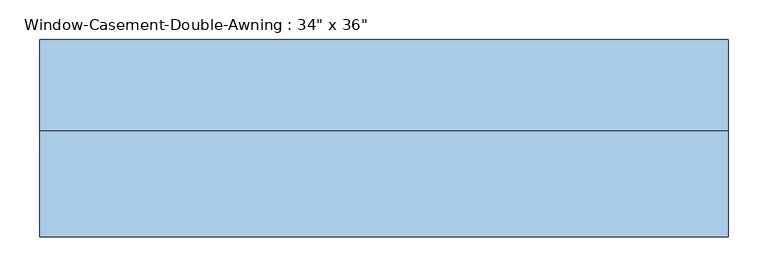
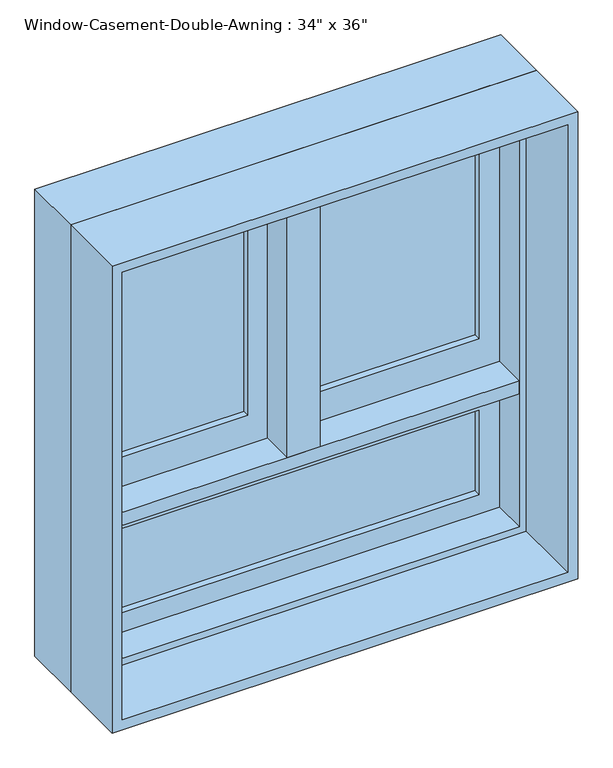
"""IFC4 building model written with IfcOpenShell, lengths in millimetres: window geometry."""

from ifc_helpers import new_model, si_unit, frame, origin, place, context, project, spatial, polyline, outline, extrude, faceted_brep, source, transform, mapped, element, save


def window_ced37e8f(model_context):
    return source(origin(), model_context, "Body", "SolidModel", [
        faceted_brep([(400.05, 82.55, 1797.05), (400.05, 19.05, 1797.05), (-400.05, 19.05, 1797.05), (-400.05, 82.55, 1797.05), (419.1, 133.35, 1816.1), (419.1, 82.55, 1816.1), (-419.1, 82.55, 1816.1), (-419.1, 133.35, 1816.1), (431.8, 19.05, 1828.8), (431.8, 133.35, 1828.8), (-431.8, 133.35, 1828.8), (-431.8, 19.05, 1828.8), (-400.05, 19.05, 946.15), (-400.05, 82.55, 946.15), (-419.1, 82.55, 927.1), (-419.1, 133.35, 927.1), (-431.8, 133.35, 914.4), (-431.8, 19.05, 914.4), (400.05, 19.05, 946.15), (400.05, 82.55, 946.15), (419.1, 82.55, 927.1), (419.1, 133.35, 927.1), (431.8, 133.35, 914.4), (431.8, 19.05, 914.4)], [[[0, 1, 2, 3]], [[4, 5, 6, 7]], [[8, 9, 10, 11]], [[3, 2, 12, 13]], [[7, 6, 14, 15]], [[11, 10, 16, 17]], [[13, 12, 18, 19]], [[15, 14, 20, 21]], [[17, 16, 22, 23]], [[11, 17, 23, 8], [1, 18, 12, 2]], [[19, 18, 1, 0]], [[5, 20, 14, 6], [3, 13, 19, 0]], [[21, 20, 5, 4]], [[23, 22, 9, 8]], [[9, 22, 16, 10], [7, 15, 21, 4]]]),
        extrude(outline(polyline([(1231.9, 419.1), (1816.1, 419.1), (1816.1, 9.525), (1231.9, 9.525), (1231.9, 419.1)]), holes=[polyline([(1289.05, 66.675), (1758.95, 66.675), (1758.95, 361.95), (1289.05, 361.95), (1289.05, 66.675)])]), frame((0.0, 82.55, 0.0), z_axis=(0.0, 1.0, 0.0), x_axis=(0.0, 0.0, 1.0)), (0.0, 0.0, 1.0), 44.45),
        extrude(outline(polyline([(1816.1, -419.1), (1231.9, -419.1), (1231.9, -9.525), (1816.1, -9.525), (1816.1, -419.1)]), holes=[polyline([(1758.95, -66.675), (1289.05, -66.675), (1289.05, -361.95), (1758.95, -361.95), (1758.95, -66.675)])]), frame((0.0, 82.55, 0.0), z_axis=(0.0, 1.0, 0.0), x_axis=(0.0, 0.0, 1.0)), (0.0, 0.0, 1.0), 44.45),
        extrude(outline(polyline([(361.95, 114.3), (361.95, 107.95), (66.675, 107.95), (66.675, 114.3), (361.95, 114.3)])), frame((0.0, 0.0, 1289.05), z_axis=(0.0, 0.0, 1.0), x_axis=(1.0, 0.0, 0.0)), (0.0, 0.0, 1.0), 469.9),
        extrude(outline(polyline([(66.675, 95.25), (66.675, 101.6), (361.95, 101.6), (361.95, 95.25), (66.675, 95.25)])), frame((0.0, 0.0, 1289.05), z_axis=(0.0, 0.0, 1.0), x_axis=(1.0, 0.0, 0.0)), (0.0, 0.0, 1.0), 469.9),
        extrude(outline(polyline([(-66.675, 114.3), (-66.675, 107.95), (-361.95, 107.95), (-361.95, 114.3), (-66.675, 114.3)])), frame((0.0, 0.0, 1289.05), z_axis=(0.0, 0.0, 1.0), x_axis=(1.0, 0.0, 0.0)), (0.0, 0.0, 1.0), 469.9),
        extrude(outline(polyline([(-361.95, 95.25), (-361.95, 101.6), (-66.675, 101.6), (-66.675, 95.25), (-361.95, 95.25)])), frame((0.0, 0.0, 1289.05), z_axis=(0.0, 0.0, 1.0), x_axis=(1.0, 0.0, 0.0)), (0.0, 0.0, 1.0), 469.9),
        extrude(outline(polyline([(400.05, 19.05), (-400.05, 19.05), (-400.05, 82.55), (-419.1, 82.55), (-419.1, 133.35), (419.1, 133.35), (419.1, 82.55), (400.05, 82.55), (400.05, 19.05)])), frame((0.0, 0.0, 1206.5), z_axis=(0.0, 0.0, 1.0), x_axis=(1.0, 0.0, 0.0)), (0.0, 0.0, 1.0), 25.4),
        extrude(outline(polyline([(1206.5, -419.1), (927.1, -419.1), (927.1, 419.1), (1206.5, 419.1), (1206.5, -419.1)]), holes=[polyline([(1149.35, 361.95), (984.25, 361.95), (984.25, -361.95), (1149.35, -361.95), (1149.35, 361.95)])]), frame((0.0, 82.55, 0.0), z_axis=(0.0, 1.0, 0.0), x_axis=(0.0, 0.0, 1.0)), (0.0, 0.0, 1.0), 44.45),
        extrude(outline(polyline([(361.95, 114.3), (361.95, 107.95), (-361.95, 107.95), (-361.95, 114.3), (361.95, 114.3)])), frame((0.0, 0.0, 984.25), z_axis=(0.0, 0.0, 1.0), x_axis=(1.0, 0.0, 0.0)), (0.0, 0.0, 1.0), 165.1),
        extrude(outline(polyline([(361.95, 101.6), (361.95, 95.25), (-361.95, 95.25), (-361.95, 101.6), (361.95, 101.6)])), frame((0.0, 0.0, 984.25), z_axis=(0.0, 0.0, 1.0), x_axis=(1.0, 0.0, 0.0)), (0.0, 0.0, 1.0), 165.1),
        extrude(outline(polyline([(1828.8, -431.8), (914.4, -431.8), (914.4, 431.8), (1828.8, 431.8), (1828.8, -431.8)]), holes=[polyline([(1809.75, 412.75), (933.45, 412.75), (933.45, -412.75), (1809.75, -412.75), (1809.75, 412.75)])]), frame((0.0, -114.3, 0.0), z_axis=(0.0, 1.0, 0.0), x_axis=(0.0, 0.0, 1.0)), (0.0, 0.0, 1.0), 133.35),
        faceted_brep([(9.525, 133.35, 1816.1), (-9.525, 133.35, 1816.1), (-9.525, 82.55, 1816.1), (9.525, 82.55, 1816.1), (9.525, 133.35, 1231.9), (9.525, 82.55, 1231.9), (30.1625, 82.55, 1231.9), (30.1625, 19.05, 1231.9), (-30.1625, 19.05, 1231.9), (-30.1625, 82.55, 1231.9), (-9.525, 82.55, 1231.9), (-9.525, 133.35, 1231.9), (-9.525, 82.55, 1797.05), (-30.1625, 82.55, 1797.05), (-30.1625, 19.05, 1797.05), (30.1625, 19.05, 1797.05), (30.1625, 82.55, 1797.05), (9.525, 82.55, 1797.05)], [[[0, 1, 2, 3]], [[4, 5, 6, 7, 8, 9, 10, 11]], [[1, 0, 4, 11]], [[2, 1, 11, 10, 12]], [[10, 9, 13, 12]], [[9, 8, 14, 13]], [[8, 7, 15, 14]], [[7, 6, 16, 15]], [[6, 5, 17, 16]], [[0, 3, 17, 5, 4]], [[12, 17, 3, 2]], [[17, 12, 13, 14, 15, 16]]]),
    ])


if __name__ == "__main__":
    model = new_model("IFC4")
    model_context = context("Model", 3, world=origin())
    ifc_project = project(units=[si_unit("LENGTHUNIT", "METRE", prefix="MILLI")], contexts=[model_context])
    site = spatial("IfcSite", under=ifc_project)
    building = spatial("IfcBuilding", under=site)
    placement = place(None, origin())
    window_shape = window_ced37e8f(model_context)
    element("IfcWindow", 1, ObjectType="Window-Casement-Double-Awning : 34\" x 36\"", at=placement, inside=building, context=model_context, shape_type="MappedRepresentation", body=[
        mapped(window_shape, transform((0.0, 0.0, 0.0), x_axis=(1.0, 0.0, 0.0), y_axis=(0.0, 1.0, 0.0), z_axis=(0.0, 0.0, 1.0))),
    ])
    save(model, "model.ifc")

# Revit data of these elements
# Type "Window-Casement-Double-Awning : 34\" x 36\""
#   Type Mark = "28"
#   Fire Rating = "0.5h"
#   Assembly Code = "B2020100"
#   Analytic Construction = "Double glazing - domestic"
#   Window Inset [instance default] = 0' - 0"
#   Wall Thickness [instance default] = 0' - 6"
#   Interior Wall Closure [instance default] = 0' - 2 1/4"
#   Half Width = 1' - 5"
#   Visual Light Transmittance = 0.81
#   Thermal Resistance (R) = 1.8146 (h·ft²·°F)/BTU
#   Solar Heat Gain Coefficient = 0.76
#   Rough Width = 2' - 10 1/2"
#   Rough Height = 3' - 0 1/2"
#   Open Window Height = 2' - 0"
#   Height = 3' - 0"
#   Heat Transfer Coefficient (U) = 0.5511 BTU/(h·ft²·°F)
#   Frame Extension [instance default] = 0' - 0 1/4"
#   Exterior Wall Closure [instance default] = 0' - 1 1/4"
#   Awning Height = 1' - 0"
#   Extension Jamb [instance default] = 0' - 2 1/4"
#   Default Sill Height = 3' - 0"
#   Width = 2' - 10"
#   Top Muntin Visibility = yes
#   Interior Trim Visibility [instance default] = yes
#   Bottom Muntin Visibility = yes
#   Exterior Trim Visibility [instance default] = yes
#   Extension Jamb Visibility [instance default] = yes
#   Interior Trim Material = Wood - Stained
#   Muntin Pattern = Muntin Pattern_2x2 : Muntin Pattern_2x2
#   Interior Trim = Trim-Window-Interior-Flat : Picture Frame
#   Interior Frame Material = Wood - Stained
#   Exterior Trim Material = Clad - White
#   Glass Panel Material = Glass
#   Exterior Trim = Trim-Window-Exterior-Flat : with Sill
#   Exterior Frame Material = Clad - White
#   Wall Closure = (empty or 0)
# Element 1 (IfcWindow, "Window-Casement-Double-Awning : 34\" x 36\"")
#   Wall Thickness = 0' - 9"
#   Extension Jamb = 0' - 5 1/4"
#   Materials on its faces: "Wood - Stained", "Glass", "Clad - White"
# Materials
#   "Wood - Stained": class "Wood", colour RGB 224 178 126, transparency 0, Cost = 0
#   "Clad - White": class "Wood", colour RGB 242 242 238, transparency 0, Cost = 0
#   "Glass": class "Glass", colour RGB 0 128 192, transparency 0.75, Description = "Soda Lime Glass", Cost = 0
